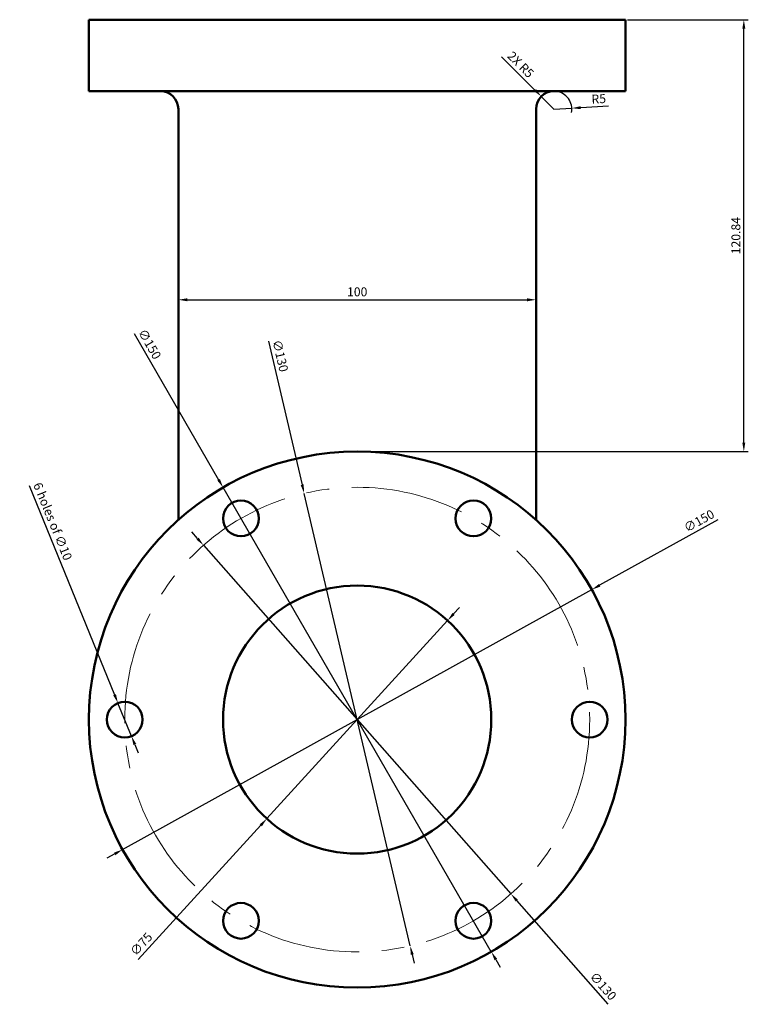
# Model space of a CAD drawing. Units: millimetres. Extents: x 1880 to 2565, y 1372 to 1704.
# Tile 2 of 2: x 2361 to 2565, y 1392 to 1667. Entities that reach past the tile are written whole.
import ezdxf

# ---------------------------------------------------------------- set-up
doc = ezdxf.new("R2010")
doc.units = ezdxf.units.MM
doc.linetypes.add('CENTER', pattern=[50.8, 31.75, -6.35, 6.35, -6.35])
for name, color, linetype, lineweight in [('M-CNTR', 4, 'CENTER', 18), ('M-DIMS', 2, 'Continuous', 25), ('M-OUTL', 7, 'Continuous', 50)]:
    doc.layers.add(name, color=color, linetype=linetype, lineweight=lineweight)
doc.styles.get("Standard").update_dxf_attribs({"font": 'arial.ttf'})
doc.dimstyles.new('ISO-25', dxfattribs={"dimtxt": 2.5, "dimasz": 2.5, "dimexe": 1.25, "dimexo": 0.625, "dimtad": 1, "dimdec": 1, "dimdsep": 46, "dimtxsty": 'Standard', "dimcen": 2.5, "dimadec": 0, "dimazin": 0, "dimtfac": 1, "dimtdec": 1, "dimtmove": 0, "dimatfit": 3, "dimfxl": 1, "dimarcsym": 0})

# ---------------------------------------------------------------- blocks, each defined once
blk = doc.blocks.new('*U1')
blk.add_circle((0, 0), 5)
blk = doc.blocks.new('*U2')
at = {"layer": 'M-OUTL', "color": 0, "linetype": 'ByBlock', "lineweight": -2, "transparency": 16777216}
for p, rotation in [((2423.17, 1527.71), 300), ((2488.17, 1527.71), 239.9999999999999), ((2520.67, 1471.41), 180), ((2423.17, 1415.12), 59.99999999999999), ((2488.17, 1415.12), 119.9999999999999)]:
    blk.add_blockref('*U1', p, dxfattribs=dict(at, rotation=rotation))
blk.add_blockref('*U1', (2390.67, 1471.41), dxfattribs=at)
blk = doc.blocks.new('*D3')
at = {"layer": 'Defpoints', "color": 0, "lineweight": 100, "transparency": 16777216}
for p in [(2510.67, 1642.25), (2515.66, 1642.5)]:
    blk.add_point(p, dxfattribs=at)
at = {"layer": 'M-DIMS', "color": 0, "lineweight": -2, "transparency": 16777216}
for p, q in [((2510.67, 1642.25), (2515.66, 1642.5)), ((2525.95, 1643.02), (2518.16, 1642.63))]:
    blk.add_line(p, q, dxfattribs=at)
blk.add_arc((2510.67, 1642.25), 5, 348.5565, 82.838, dxfattribs=at)
at = {"layer": 'M-DIMS', "color": 0, "lineweight": 100, "transparency": 16777216}
blk.add_solid([(2518.14, 1643.05), (2518.18, 1642.21), (2515.66, 1642.5)], dxfattribs=at)
at = {"layer": 'M-DIMS', "color": 0, "transparency": 16777216, "insert": (2523.21, 1644.78), "char_height": 2.5, "attachment_point": 5, "rotation": 2.8805}
blk.add_mtext('R5', dxfattribs=at)
blk = doc.blocks.new('*D4')
at = {"layer": 'Defpoints', "color": 0, "lineweight": 100, "transparency": 16777216}
for p in [(2505.67, 1588.88), (2405.67, 1584.78), (2505.67, 1584.78)]:
    blk.add_point(p, dxfattribs=at)
at = {"layer": 'M-DIMS', "color": 0, "lineweight": -2, "transparency": 16777216}
for p, q in [((2405.67, 1585.41), (2405.67, 1590.13)), ((2505.67, 1585.41), (2505.67, 1590.13)), ((2408.17, 1588.88), (2503.17, 1588.88))]:
    blk.add_line(p, q, dxfattribs=at)
at = {"layer": 'M-DIMS', "color": 0, "lineweight": 100, "transparency": 16777216}
for points in [[(2408.17, 1589.3), (2408.17, 1588.46), (2405.67, 1588.88)], [(2503.17, 1589.3), (2503.17, 1588.46), (2505.67, 1588.88)]]:
    blk.add_solid(points, dxfattribs=at)
at = {"layer": 'M-DIMS', "color": 0, "transparency": 16777216, "insert": (2455.67, 1590.78), "char_height": 2.5, "attachment_point": 5}
blk.add_mtext('100', dxfattribs=at)
blk = doc.blocks.new('*D5')
at = {"layer": 'Defpoints', "color": 0, "lineweight": 100, "transparency": 16777216}
for p in [(2521.26, 1507.78), (2390.07, 1435.05)]:
    blk.add_point(p, dxfattribs=at)
at = {"layer": 'M-DIMS', "color": 0, "lineweight": -2, "transparency": 16777216}
for p, q in [((2556.51, 1527.31), (2523.45, 1508.99)), ((2390.07, 1435.05), (2521.26, 1507.78)), ((2387.88, 1433.84), (2385.7, 1432.63))]:
    blk.add_line(p, q, dxfattribs=at)
at = {"layer": 'M-DIMS', "color": 0, "lineweight": 100, "transparency": 16777216}
for points in [[(2523.25, 1509.35), (2523.65, 1508.62), (2521.26, 1507.78)], [(2387.68, 1434.21), (2388.09, 1433.48), (2390.07, 1435.05)]]:
    blk.add_solid(points, dxfattribs=at)
at = {"layer": 'M-DIMS', "color": 0, "transparency": 16777216, "insert": (2551.41, 1526.74), "char_height": 2.5, "attachment_point": 5, "rotation": 29.0004}
blk.add_mtext('∅150', dxfattribs=at)
blk = doc.blocks.new('*D6')
at = {"layer": 'Defpoints', "color": 0, "lineweight": 100, "transparency": 16777216}
for p in [(2412.69, 1520.18), (2498.64, 1422.65)]:
    blk.add_point(p, dxfattribs=at)
at = {"layer": 'M-DIMS', "color": 0, "lineweight": -2, "transparency": 16777216}
for p, q in [((2411.04, 1522.06), (2409.39, 1523.93)), ((2412.69, 1520.18), (2498.64, 1422.65)), ((2525.87, 1391.75), (2500.3, 1420.77))]:
    blk.add_line(p, q, dxfattribs=at)
at = {"layer": 'M-DIMS', "color": 0, "lineweight": 100, "transparency": 16777216}
for points in [[(2411.35, 1522.33), (2410.73, 1521.78), (2412.69, 1520.18)], [(2500.61, 1421.05), (2499.98, 1420.5), (2498.64, 1422.65)]]:
    blk.add_solid(points, dxfattribs=at)
at = {"layer": 'M-DIMS', "color": 0, "transparency": 16777216, "insert": (2524.21, 1396.62), "char_height": 2.5, "attachment_point": 5, "rotation": 311.3888}
blk.add_mtext('∅130', dxfattribs=at)
blk = doc.blocks.new('*D7')
at = {"layer": 'Defpoints', "color": 0, "lineweight": 100, "transparency": 16777216}
for p in [(2480.93, 1499.13), (2430.4, 1443.7)]:
    blk.add_point(p, dxfattribs=at)
at = {"layer": 'M-DIMS', "color": 0, "lineweight": -2, "transparency": 16777216}
for p, q in [((2482.61, 1500.97), (2484.3, 1502.82)), ((2480.93, 1499.13), (2430.4, 1443.7)), ((2394.44, 1404.25), (2428.72, 1441.85))]:
    blk.add_line(p, q, dxfattribs=at)
at = {"layer": 'M-DIMS', "color": 0, "lineweight": 100, "transparency": 16777216}
for points in [[(2482.31, 1501.25), (2482.92, 1500.69), (2480.93, 1499.13)], [(2428.41, 1442.13), (2429.03, 1441.57), (2430.4, 1443.7)]]:
    blk.add_solid(points, dxfattribs=at)
at = {"layer": 'M-DIMS', "color": 0, "transparency": 16777216, "insert": (2395.53, 1408.38), "char_height": 2.5, "attachment_point": 5, "rotation": 47.647}
blk.add_mtext('∅75', dxfattribs=at)
blk = doc.blocks.new('*D8')
at = {"layer": 'Defpoints', "color": 0, "lineweight": 100, "transparency": 16777216}
for p in [(2388.78, 1476.04), (2392.55, 1466.78)]:
    blk.add_point(p, dxfattribs=at)
at = {"layer": 'M-DIMS', "color": 0, "lineweight": -2, "transparency": 16777216}
for p, q in [((2363.96, 1536.96), (2387.84, 1478.36)), ((2392.55, 1466.78), (2388.78, 1476.04)), ((2393.5, 1464.47), (2394.44, 1462.15))]:
    blk.add_line(p, q, dxfattribs=at)
at = {"layer": 'M-DIMS', "color": 0, "lineweight": 100, "transparency": 16777216}
for points in [[(2388.22, 1478.52), (2387.45, 1478.2), (2388.78, 1476.04)], [(2393.88, 1464.63), (2393.11, 1464.31), (2392.55, 1466.78)]]:
    blk.add_solid(points, dxfattribs=at)
at = {"layer": 'M-DIMS', "color": 0, "transparency": 16777216, "insert": (2370.25, 1526.75), "char_height": 2.5, "attachment_point": 5, "rotation": 292.1692}
blk.add_mtext('6 holes of ∅10', dxfattribs=at)
blk = doc.blocks.new('FLANGE-150x20-EDGE')
for p, q in [((0, 20), (150, 20)), ((0, 20), (0, 0)), ((150, 0), (150, 20)), ((0, 0), (150, 0))]:
    blk.add_line(p, q)
blk = doc.blocks.new('*D16')
at = {"layer": 'Defpoints', "color": 0, "lineweight": 100, "transparency": 16777216}
for p in [(2530.67, 1667.25), (2563.77, 1667.25), (2455.67, 1546.41)]:
    blk.add_point(p, dxfattribs=at)
at = {"layer": 'M-DIMS', "color": 0, "lineweight": -2, "transparency": 16777216}
for p, q in [((2531.29, 1667.25), (2565.02, 1667.25)), ((2563.77, 1548.91), (2563.77, 1664.75)), ((2456.29, 1546.41), (2565.02, 1546.41))]:
    blk.add_line(p, q, dxfattribs=at)
at = {"layer": 'M-DIMS', "color": 0, "lineweight": 100, "transparency": 16777216}
for points in [[(2563.35, 1664.75), (2564.18, 1664.75), (2563.77, 1667.25)], [(2563.35, 1548.91), (2564.18, 1548.91), (2563.77, 1546.41)]]:
    blk.add_solid(points, dxfattribs=at)
at = {"layer": 'M-DIMS', "color": 0, "transparency": 16777216, "insert": (2561.87, 1606.83), "char_height": 2.5, "attachment_point": 5, "rotation": 90}
blk.add_mtext('120.84', dxfattribs=at)
blk = doc.blocks.new('*D24')
at = {"layer": 'Defpoints', "color": 0, "lineweight": 100, "transparency": 16777216}
for p in [(2418.17, 1536.37), (2493.17, 1406.46)]:
    blk.add_point(p, dxfattribs=at)
at = {"layer": 'M-DIMS', "color": 0, "lineweight": -2, "transparency": 16777216}
for p, q in [((2393.3, 1579.44), (2416.92, 1538.53)), ((2493.17, 1406.46), (2418.17, 1536.37)), ((2494.42, 1404.3), (2495.67, 1402.13))]:
    blk.add_line(p, q, dxfattribs=at)
at = {"layer": 'M-DIMS', "color": 0, "lineweight": 100, "transparency": 16777216}
for points in [[(2417.28, 1538.74), (2416.56, 1538.32), (2418.17, 1536.37)], [(2494.78, 1404.51), (2494.06, 1404.09), (2493.17, 1406.46)]]:
    blk.add_solid(points, dxfattribs=at)
at = {"layer": 'M-DIMS', "color": 0, "transparency": 16777216, "insert": (2397.37, 1576.32), "char_height": 2.5, "attachment_point": 5, "rotation": 299.9998}
blk.add_mtext('∅150', dxfattribs=at)
blk = doc.blocks.new('*D25')
at = {"layer": 'Defpoints', "color": 0, "lineweight": 100, "transparency": 16777216}
for p in [(2440.85, 1534.7), (2470.48, 1408.13)]:
    blk.add_point(p, dxfattribs=at)
at = {"layer": 'M-DIMS', "color": 0, "lineweight": -2, "transparency": 16777216}
for p, q in [((2430.88, 1577.29), (2440.28, 1537.14)), ((2470.48, 1408.13), (2440.85, 1534.7)), ((2471.05, 1405.69), (2471.62, 1403.26))]:
    blk.add_line(p, q, dxfattribs=at)
at = {"layer": 'M-DIMS', "color": 0, "lineweight": 100, "transparency": 16777216}
for points in [[(2440.69, 1537.23), (2439.87, 1537.04), (2440.85, 1534.7)], [(2471.46, 1405.79), (2470.65, 1405.6), (2470.48, 1408.13)]]:
    blk.add_solid(points, dxfattribs=at)
at = {"layer": 'M-DIMS', "color": 0, "transparency": 16777216, "insert": (2433.88, 1573.13), "char_height": 2.5, "attachment_point": 5, "rotation": 283.177}
blk.add_mtext('∅130', dxfattribs=at)
blk = doc.blocks.new('*D26')
at = {"layer": 'Defpoints', "color": 0, "lineweight": 100, "transparency": 16777216}
for p in [(2507.13, 1645.79), (2510.67, 1642.25)]:
    blk.add_point(p, dxfattribs=at)
at = {"layer": 'M-DIMS', "color": 0, "lineweight": -2, "transparency": 16777216}
for p, q in [((2496.02, 1656.9), (2505.36, 1647.56)), ((2510.67, 1642.25), (2507.13, 1645.79))]:
    blk.add_line(p, q, dxfattribs=at)
at = {"layer": 'M-DIMS', "color": 0, "lineweight": 100, "transparency": 16777216}
blk.add_solid([(2505.66, 1647.85), (2505.07, 1647.26), (2507.13, 1645.79)], dxfattribs=at)
at = {"layer": 'M-DIMS', "color": 0, "transparency": 16777216, "insert": (2501.15, 1654.46), "char_height": 2.5, "attachment_point": 5, "rotation": 315.0051}
blk.add_mtext('2X R5', dxfattribs=at)

msp = doc.modelspace()

# ---------------------------------------------------------------- linework, layer by layer
at = {"layer": 'M-CNTR'}
msp.add_circle((2455.667, 1471.414), 65, dxfattribs=at)
at = {"layer": 'M-OUTL'}
for p, q in [((2530.667, 1667.253), (2530.667, 1647.253)), ((2400.667, 1647.253), (2380.667, 1647.253)), ((2530.667, 1647.253), (2510.667, 1647.253)), ((2405.667, 1527.316), (2405.667, 1642.253)), ((2505.667, 1527.316), (2505.667, 1642.253))]:
    msp.add_line(p, q, dxfattribs=at)
for radius in [75, 37.5]:
    msp.add_circle((2455.667, 1471.414), radius, dxfattribs=at)
for centre, start, end in [((2400.667, 1642.253), 0, 90), ((2510.667, 1642.253), 90, 180)]:
    msp.add_arc(centre, 5, start, end, dxfattribs=at)

# ---------------------------------------------------------------- block references
at = {"layer": 'M-OUTL', "rotation": 180}
msp.add_blockref('FLANGE-150x20-EDGE', (2530.667, 1667.252), dxfattribs=at)
at = {"layer": 'M-OUTL'}
msp.add_blockref('*U2', (0, 0), dxfattribs=at)

# ---------------------------------------------------------------- dimensions: what is measured, and where the dimension line sits
at = {"layer": 'M-DIMS'}
dim = msp.add_linear_dim(base=(2563.767, 1667.253), p1=(2455.667, 1546.414), p2=(2530.667, 1667.253), angle=90, dimstyle='ISO-25', override={"dimdec": 2, "dimlfac": 1, "dimrnd": 0, "dimzin": 0, "dimdsep": 46, "dimlunit": 2}, dxfattribs=at)
dim.commit()
dim.dimension.update_dxf_attribs({"geometry": '*D16', "text_midpoint": (2561.865, 1606.833)})
dim = msp.add_radius_dim(center=(2510.667, 1642.253), mpoint=(2507.131, 1645.788), text='2X <>', dimstyle='ISO-25', override={"dimdec": 0, "dimlfac": 1, "dimrnd": 0, "dimzin": 0, "dimdsep": 46, "dimlunit": 2}, dxfattribs=at)
dim.commit()
dim.dimension.update_dxf_attribs({"geometry": '*D26', "text_midpoint": (2501.151, 1654.456)})
dim = msp.add_radius_dim(center=(2510.667, 1642.253), mpoint=(2515.66, 1642.504), dimstyle='ISO-25', override={"dimclrd": 0, "dimclre": 0, "dimclrt": 0}, dxfattribs=at)
dim.commit()
dim.dimension.update_dxf_attribs({"geometry": '*D3', "text_midpoint": (2523.206, 1644.782)})
dim = msp.add_linear_dim(base=(2505.667, 1588.879), p1=(2405.667, 1584.784), p2=(2505.667, 1584.784), dimstyle='ISO-25', override={"dimclrd": 0, "dimclre": 0, "dimclrt": 0}, dxfattribs=at)
dim.commit()
dim.dimension.update_dxf_attribs({"geometry": '*D4', "text_midpoint": (2455.667, 1590.78)})
for p1, p2, override, picture, middle in [((2493.167, 1406.462), (2418.167, 1536.366), {"dimdec": 0, "dimlfac": 1, "dimrnd": 0, "dimzin": 0, "dimdsep": 46, "dimlunit": 2}, '*D24', (2395.667, 1575.337)), ((2470.484, 1408.125), (2440.849, 1534.703), {"dimdec": 0, "dimlfac": 1, "dimrnd": 0, "dimzin": 0, "dimdsep": 46, "dimlunit": 2}, '*D25', (2431.959, 1572.676)), ((2390.071, 1435.053), (2521.263, 1507.775), {"dimclrd": 0, "dimclre": 0, "dimclrt": 0}, '*D5', (2552.363, 1525.014)), ((2412.691, 1520.18), (2498.643, 1422.648), {"dimclrd": 0, "dimclre": 0, "dimclrt": 0}, '*D6', (2522.733, 1395.312)), ((2480.93, 1499.127), (2430.403, 1443.701), {"dimclrd": 0, "dimclre": 0, "dimclrt": 0}, '*D7', (2396.989, 1407.048))]:
    dim = msp.add_diameter_dim_2p(p1=p1, p2=p2, dimstyle='ISO-25', override=override, dxfattribs=at)
    dim.commit()
    dim.dimension.update_dxf_attribs({"geometry": picture, "text_midpoint": middle, "dimtype": 163})
dim = msp.add_diameter_dim_2p(p1=(2392.553, 1466.784), p2=(2388.78, 1476.044), text='6 holes of <>', dimstyle='ISO-25', override={"dimclrd": 0, "dimclre": 0, "dimclrt": 0}, dxfattribs=at)
dim.commit()
dim.dimension.update_dxf_attribs({"geometry": '*D8', "text_midpoint": (2368.423, 1526.005), "dimtype": 163})

doc.saveas('drawing.dxf')
